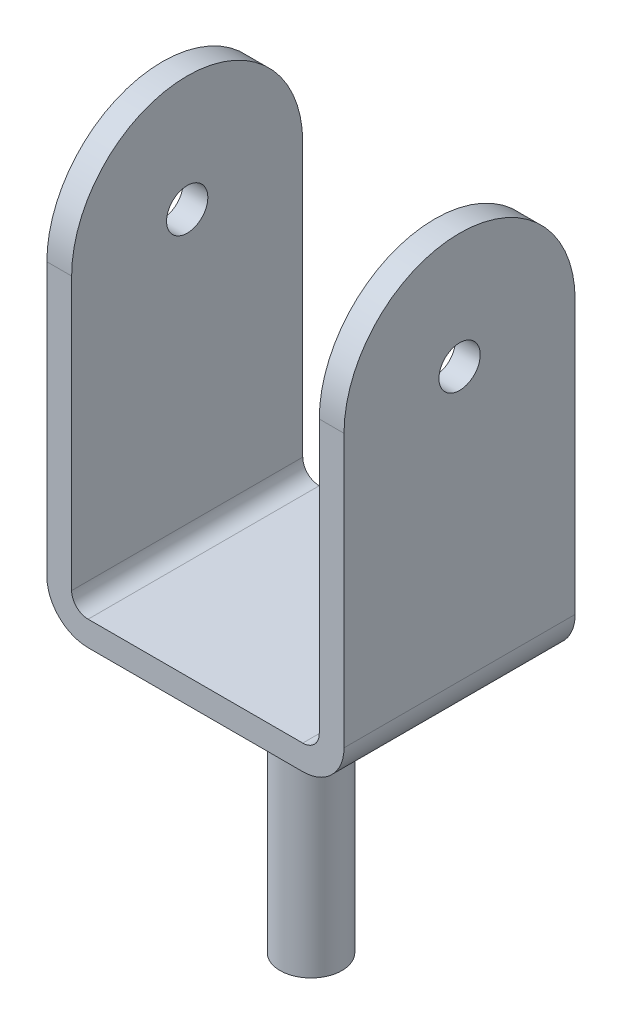
from build123d import *

# Parameters (mm, degrees)
U_CHANNEL_BODY_DEPTH                  = 140
ROUNDED_ENDS_AND_PIN_HOLES_DEPTH      = 568.802782663
ROUNDED_ENDS_AND_PIN_HOLES_DEPTH_BACK = 568.802782663
ROUNDED_ENDS_AND_PIN_HOLE_SKETCH_R    = 25
SHANK_PROFILE_SKETCH_R                = 37.5
ROUND_SHANK_DEPTH                     = 355


with BuildPart() as part:
    # U-Channel Profile Sketch → U-Channel Body (new, symmetric)
    with BuildSketch(Plane.XY):
        with BuildLine():
            Line((-180, 520), (-180, 50))
            ThreePointArc((-180, 50), (-165.355339059, 14.644660941), (-130, 0))
            Line((-130, 0), (130, 0))
            ThreePointArc((130, 0), (165.355339059, 14.644660941), (180, 50))
            Line((180, 50), (180, 520))
            Line((180, 520), (150, 520))
            Line((150, 520), (150, 50))
            ThreePointArc((150, 50), (144.142135624, 35.857864376), (130, 30))
            Line((130, 30), (-130, 30))
            ThreePointArc((-130, 30), (-144.142135624, 35.857864376), (-150, 50))
            Line((-150, 50), (-150, 520))
            Line((-150, 520), (-180, 520))
        make_face()
    extrude(amount=U_CHANNEL_BODY_DEPTH, both=True)

    # Rounded Ends and Pin Hole Sketch → Rounded Ends and Pin Holes (cut, two sides: drawn at the far end of the back side and taken through both)
    with BuildSketch(Plane(origin=(0, 0, 0), x_dir=(0, 0, -1), z_dir=(1, 0, 0)).offset(-ROUNDED_ENDS_AND_PIN_HOLES_DEPTH_BACK)):
        with BuildLine():
            Line((-6.91e-07, 520), (-140, 520))
            Line((-140, 520), (-140, 380))
            ThreePointArc((-140, 380), (-98.99494961, 478.994949122), (-6.91e-07, 520))
        make_face()
        with BuildLine():
            Line((140, 520), (-6.91e-07, 520))
            ThreePointArc((-6.91e-07, 520), (98.994949122, 478.99494961), (140, 380))
            Line((140, 380), (140, 520))
        make_face()
        with Locations((0, 380)):
            Circle(ROUNDED_ENDS_AND_PIN_HOLE_SKETCH_R)
    extrude(amount=ROUNDED_ENDS_AND_PIN_HOLES_DEPTH + ROUNDED_ENDS_AND_PIN_HOLES_DEPTH_BACK, mode=Mode.SUBTRACT)

    # Shank Profile Sketch → Round Shank (add)
    with BuildSketch(Plane(origin=(0, 30, 0), x_dir=(1, 0, 0), z_dir=(0, 1, 0))):
        with Locations(Location((0, 0, 0), (0, 0, 270))):
            Circle(SHANK_PROFILE_SKETCH_R)
    extrude(amount=-ROUND_SHANK_DEPTH)


solid = part.part
